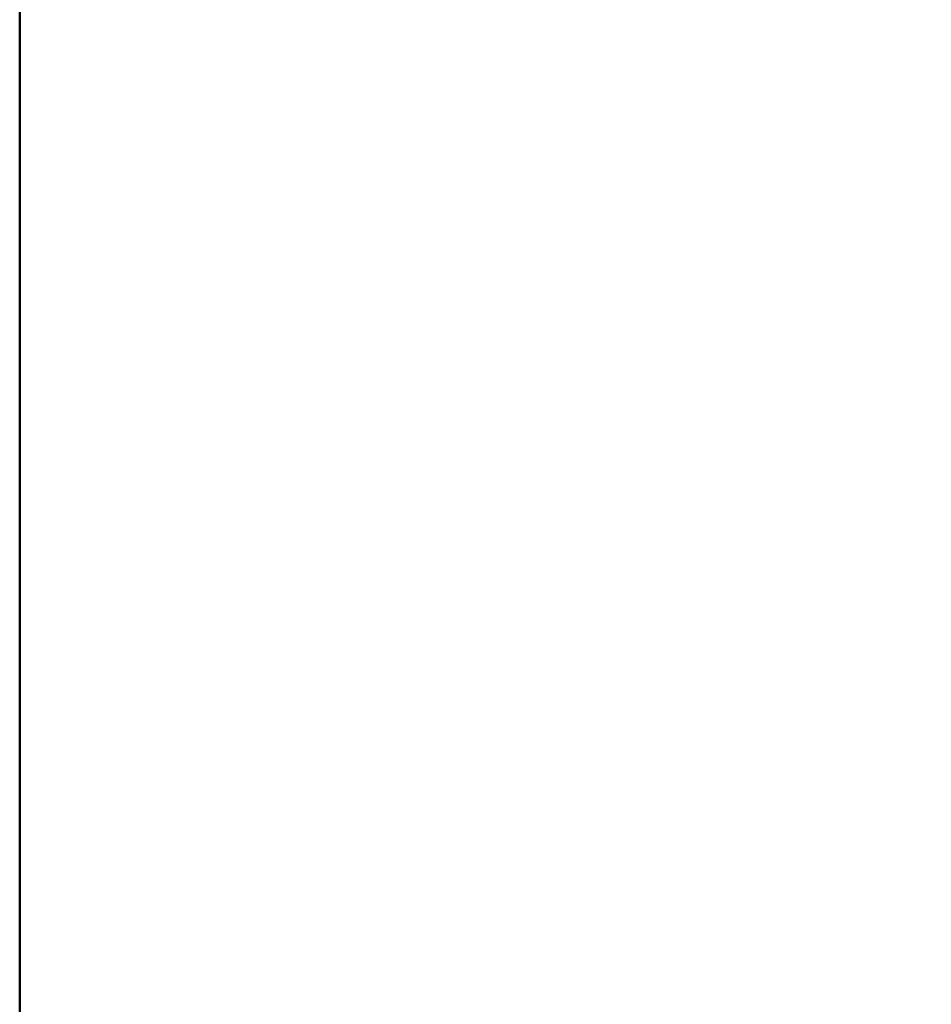
# Model space of a CAD drawing. Units: inches. Extents: x 64 to 1167, y 117 to 939.
# Tile 6 of 56: x 64 to 121, y 583 to 644. Entities that reach past the tile are written whole.
import ezdxf

# ---------------------------------------------------------------- set-up
doc = ezdxf.new("R2010")
doc.units = ezdxf.units.IN
doc.header["$MEASUREMENT"] = 0
doc.layers.add('A-ANNO-TTLB', color=7, linetype='Continuous', lineweight=50)

msp = doc.modelspace()

# ---------------------------------------------------------------- linework, layer by layer
at = {"layer": 'A-ANNO-TTLB'}
msp.add_lwpolyline([(64.30944150321102, 939.2206678261972), (512.7662400313202, 939.2206678261972), (512.7662400313202, 116.5466470696337), (64.30944150321102, 116.5466470696337)], close=True, dxfattribs=at)

doc.saveas('drawing.dxf')
